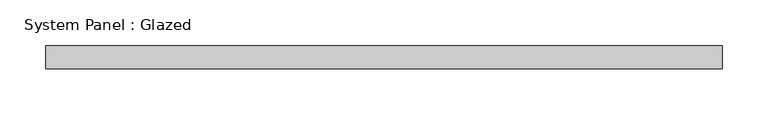
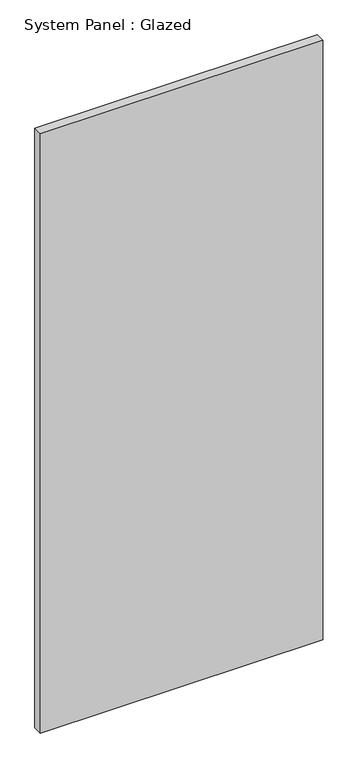
"""IFC4 building model written with IfcOpenShell, lengths in millimetres: plate geometry, System Panel : Glazed."""

from ifc_helpers import new_model, si_unit, origin, origin_with_axes, place, context, project, spatial, polyline, outline, extrude, source, transform, mapped, element, save


def system_panel_glazed_c6240b01(model_context):
    return source(origin(), model_context, "Body", "SweptSolid", [
        extrude(outline(polyline([(371.475, 19.05), (-371.475, 19.05), (-371.475, 44.45), (371.475, 44.45), (371.475, 19.05)])), origin_with_axes(), (0.0, 0.0, 1.0), 1665.8537153),
    ])


if __name__ == "__main__":
    model = new_model("IFC4")
    model_context = context("Model", 3, world=origin())
    ifc_project = project(units=[si_unit("LENGTHUNIT", "METRE", prefix="MILLI")], contexts=[model_context])
    site = spatial("IfcSite", under=ifc_project)
    building = spatial("IfcBuilding", under=site)
    placement = place(None, origin())
    system_panel_glazed_shape = system_panel_glazed_c6240b01(model_context)
    element("IfcPlate", 1, ObjectType="System Panel : Glazed", at=placement, inside=building, context=model_context, shape_type="MappedRepresentation", body=[
        mapped(system_panel_glazed_shape, transform((0.0, 0.0, 0.0), x_axis=(1.0, 0.0, 0.0), y_axis=(0.0, 1.0, 0.0), z_axis=(0.0, 0.0, 1.0))),
    ])
    save(model, "model.ifc")

# Revit data of these elements
# Type "System Panel : Glazed"
#   Construction Type Id = "GSP4R"
#   Analytic Construction = "1/8 in Pilkington single glazing"
#   Visual Light Transmittance = 0.9
#   Solar Heat Gain Coefficient = 0.86
#   Heat Transfer Coefficient (U) = 1.18115 BTU/(h·ft²·°F)
#   Define Thermal Properties by = 1
# Element 1 (IfcPlate, "System Panel : Glazed")
#   Materials on its faces: "Glass"
# Materials
#   "Glass": class "Glass", colour RGB 0 128 192, transparency 0.75, Description = "Soda Lime Glass", Cost = 0
